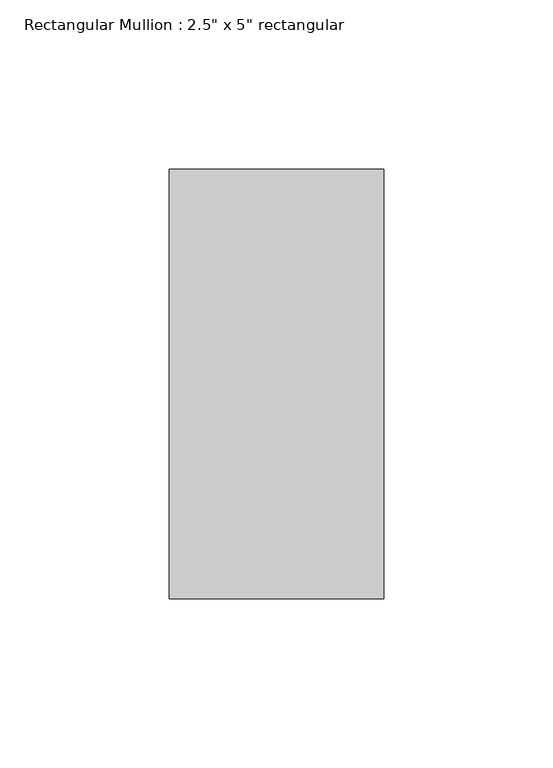
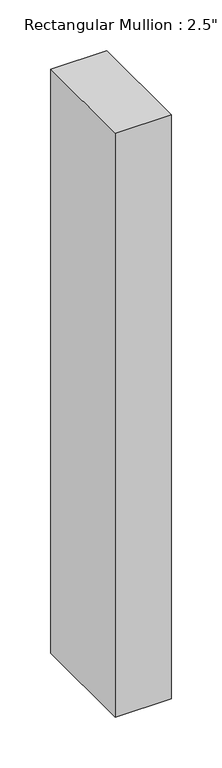
"""IFC4 building model written with IfcOpenShell, lengths in millimetres: member geometry."""

from ifc_helpers import new_model, si_unit, frame, origin, place, context, project, spatial, polyline, outline, extrude, source, transform, mapped, element, save


def member_db897065(model_context):
    return source(origin(), model_context, "Body", "SweptSolid", [
        extrude(outline(polyline([(31.75, 63.5), (31.75, -63.5), (-31.75, -63.5), (-31.75, 63.5), (31.75, 63.5)])), frame((0.0, 0.0, -702.226051), z_axis=(0.0, 0.0, 1.0), x_axis=(1.0, 0.0, 0.0)), (0.0, 0.0, 1.0), 702.226051),
    ])


if __name__ == "__main__":
    model = new_model("IFC4")
    model_context = context("Model", 3, world=origin())
    ifc_project = project(units=[si_unit("LENGTHUNIT", "METRE", prefix="MILLI")], contexts=[model_context])
    site = spatial("IfcSite", under=ifc_project)
    building = spatial("IfcBuilding", under=site)
    placement = place(None, origin())
    member_shape = member_db897065(model_context)
    element("IfcMember", 1, ObjectType="Rectangular Mullion : 2.5\" x 5\" rectangular", at=placement, inside=building, context=model_context, shape_type="MappedRepresentation", body=[
        mapped(member_shape, transform((0.0, 0.0, 0.0), x_axis=(1.0, 0.0, 0.0), y_axis=(0.0, 1.0, 0.0), z_axis=(0.0, 0.0, 1.0))),
    ])
    save(model, "model.ifc")

# Revit data of these elements
# Type "Rectangular Mullion : 2.5\" x 5\" rectangular"
#   built-in parameter 1007304 = 0.416667 (stored number, unit not read)
#   built-in parameter 1007301 = 0.104167 (stored number, unit not read)
#   built-in parameter 1007300 = 0.104167 (stored number, unit not read)
# Element 1 (IfcMember, "Rectangular Mullion : 2.5\" x 5\" rectangular")
#   Materials on its faces: "Aluminum"
# Materials
#   "Aluminum": class "Metal", colour RGB 247 247 247, transparency 0, Description = "Aluminum 6061", Cost = 0
